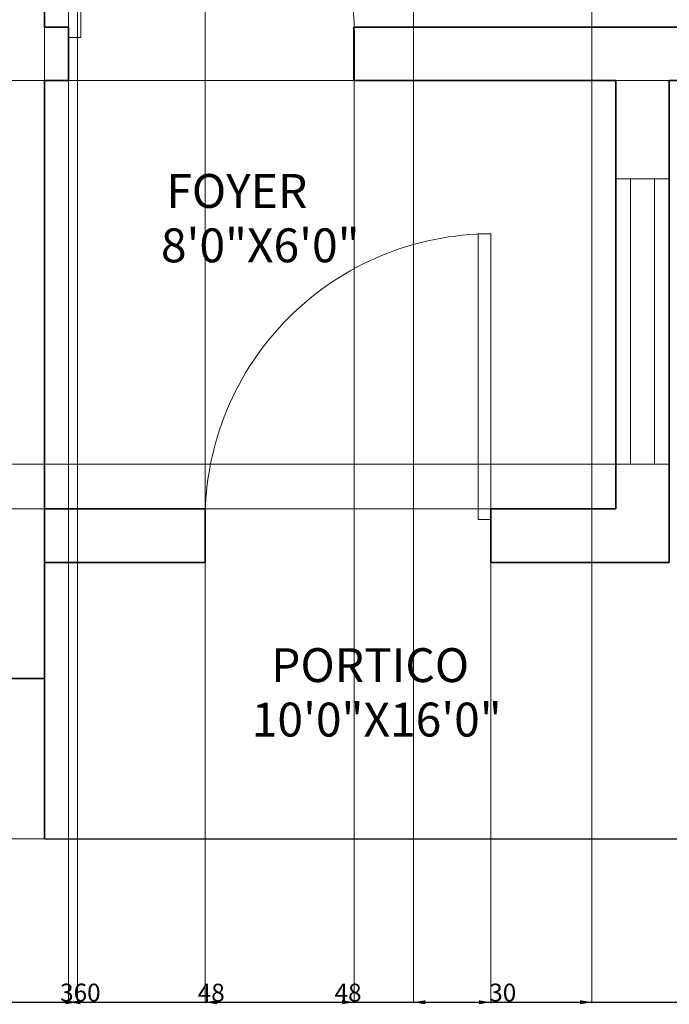
# Model space of a CAD drawing. Units: feet. Extents: x -297 to 770, y -228 to 625.
# Tile 3 of 14: x 552 to 661, y -228 to -62. Entities that reach past the tile are written whole.
import ezdxf

# ---------------------------------------------------------------- set-up
doc = ezdxf.new("R2010")
doc.units = ezdxf.units.FT
doc.header["$MEASUREMENT"] = 0
for name, color, linetype, lineweight in [('A-ANNO-DIMS', 2, 'Continuous', 18), ('A-AREA-IDEN', 7, 'Continuous', 25), ('A-FLOR-EDGE', 7, 'Continuous', 25), ('A-WALL', 7, 'Continuous', 35), ('doors', 30, 'Continuous', 18), ('windows', 30, 'Continuous', 18)]:
    doc.layers.add(name, color=color, linetype=linetype, lineweight=lineweight)
doc.styles.add('Annotative', font='arial.ttf')
doc.styles.get("Standard").update_dxf_attribs({"font": 'arial.ttf'})
doc.dimstyles.get("Standard").update_dxf_attribs({"dimtxt": 3, "dimasz": 2, "dimexe": 0.18, "dimexo": 0.0625, "dimgap": 0.09, "dimtad": 1, "dimtoh": 1, "dimdec": 1, "dimzin": 0, "dimdsep": 46, "dimlunit": 3, "dimtxsty": 'Standard', "dimcen": 0, "dimclre": 256, "dimadec": 0, "dimazin": 0, "dimtfac": 1, "dimtdec": 1, "dimtofl": 0, "dimtmove": 0, "dimatfit": 3, "dimfxl": 1, "dimtolj": 1, "dimtzin": 0, "dimlwe": -1, "dimarcsym": 0})

# ---------------------------------------------------------------- blocks, each defined once
blk = doc.blocks.new('*U5')
for p, q in [((-40, 0), (-40, 6)), ((0, 0), (0, 6))]:
    blk.add_line(p, q)
blk.add_lwpolyline([(0, 0), (0, -40), (-1.75, -40), (-1.75, 0)], close=True)
blk.add_arc((0, 0), 40, 180, 270)
blk = doc.blocks.new('*U4')
for p, q in [((0, 0), (0, 6)), ((40, 0), (40, 6))]:
    blk.add_line(p, q)
blk.add_lwpolyline([(0, 0), (0, -40), (1.75, -40), (1.75, 0)], close=True)
blk.add_arc((0, 0), 40, 270, 0)
blk = doc.blocks.new('WIN-4FT')
for p, q in [((48, 9), (0, 9)), ((0, 9), (0, 0)), ((48, 0), (48, 9)), ((0, 6.5), (48, 6.5)), ((0, 2.5), (48, 2.5)), ((0, 0), (48, 0))]:
    blk.add_line(p, q)
blk = doc.blocks.new('*D43')
at = {"layer": 'A-ANNO-DIMS', "transparency": 16777216}
for p, q in [((382.16, -173.1), (382.16, -227.67)), ((742.16, -200.1), (742.16, -227.67))]:
    blk.add_line(p, q, dxfattribs=at)
at = {"layer": 'A-ANNO-DIMS', "color": 0, "lineweight": -2, "transparency": 16777216}
blk.add_line((384.16, -227.49), (740.16, -227.49), dxfattribs=at)
at = {"layer": 'A-ANNO-DIMS', "color": 0, "transparency": 16777216}
for points in [[(384.16, -227.15), (384.16, -227.82), (382.16, -227.49)], [(740.16, -227.15), (740.16, -227.82), (742.16, -227.49)]]:
    blk.add_solid(points, dxfattribs=at)
at = {"layer": 'Defpoints', "color": 0, "transparency": 16777216}
for p in [(382.16, -173.04), (742.16, -200.04), (742.16, -227.49)]:
    blk.add_point(p, dxfattribs=at)
at = {"layer": 'A-ANNO-DIMS', "color": 0, "transparency": 16777216, "insert": (562.16, -225.86), "char_height": 3, "attachment_point": 5}
blk.add_mtext('\\A1;360', dxfattribs=at)
blk = doc.blocks.new('*D45')
at = {"layer": 'A-ANNO-DIMS', "transparency": 16777216}
for p, q in [((382.09, -173.04), (354.53, -173.04)), ((556.09, -200.04), (354.53, -200.04))]:
    blk.add_line(p, q, dxfattribs=at)
at = {"layer": 'A-ANNO-DIMS', "color": 0, "lineweight": -2, "transparency": 16777216}
blk.add_line((354.71, -175.04), (354.71, -198.04), dxfattribs=at)
at = {"layer": 'A-ANNO-DIMS', "color": 0, "transparency": 16777216}
for points in [[(354.37, -175.04), (355.04, -175.04), (354.71, -173.04)], [(354.37, -198.04), (355.04, -198.04), (354.71, -200.04)]]:
    blk.add_solid(points, dxfattribs=at)
at = {"layer": 'Defpoints', "color": 0, "transparency": 16777216}
for p in [(382.16, -173.04), (354.71, -200.04), (556.16, -200.04)]:
    blk.add_point(p, dxfattribs=at)
at = {"layer": 'A-ANNO-DIMS', "color": 0, "transparency": 16777216, "insert": (353.11, -186.54), "char_height": 3, "attachment_point": 5, "rotation": 90}
blk.add_mtext('\\A1;27', dxfattribs=at)
blk = doc.blocks.new('*D56')
at = {"layer": 'A-ANNO-DIMS', "transparency": 16777216}
for p, q in [((742.09, -72.54), (354.53, -72.54)), ((742.09, -200.04), (354.53, -200.04))]:
    blk.add_line(p, q, dxfattribs=at)
at = {"layer": 'A-ANNO-DIMS', "color": 0, "lineweight": -2, "transparency": 16777216}
blk.add_line((354.71, -74.54), (354.71, -198.04), dxfattribs=at)
at = {"layer": 'A-ANNO-DIMS', "color": 0, "transparency": 16777216}
for points in [[(354.37, -74.54), (355.04, -74.54), (354.71, -72.54)], [(354.37, -198.04), (355.04, -198.04), (354.71, -200.04)]]:
    blk.add_solid(points, dxfattribs=at)
at = {"layer": 'Defpoints', "color": 0, "transparency": 16777216}
for p in [(742.16, -72.54), (354.71, -200.04), (742.16, -200.04)]:
    blk.add_point(p, dxfattribs=at)
at = {"layer": 'A-ANNO-DIMS', "color": 0, "transparency": 16777216, "insert": (353.08, -136.29), "char_height": 3, "attachment_point": 5, "rotation": 90}
blk.add_mtext('\\A1;127.5', dxfattribs=at)
blk = doc.blocks.new('*D59')
at = {"layer": 'A-ANNO-DIMS', "transparency": 16777216}
for p, q in [((652.09, -137.04), (354.53, -137.04)), ((652.09, -144.54), (354.53, -144.54))]:
    blk.add_line(p, q, dxfattribs=at)
at = {"layer": 'A-ANNO-DIMS', "color": 0, "lineweight": -2, "transparency": 16777216}
blk.add_line((354.71, -142.54), (354.71, -139.04), dxfattribs=at)
at = {"layer": 'A-ANNO-DIMS', "color": 0, "transparency": 16777216}
for points in [[(354.37, -139.04), (355.04, -139.04), (354.71, -137.04)], [(354.37, -142.54), (355.04, -142.54), (354.71, -144.54)]]:
    blk.add_solid(points, dxfattribs=at)
at = {"layer": 'Defpoints', "color": 0, "transparency": 16777216}
for p in [(354.71, -137.04), (652.16, -137.04), (652.16, -144.54)]:
    blk.add_point(p, dxfattribs=at)
at = {"layer": 'A-ANNO-DIMS', "color": 0, "transparency": 16777216, "insert": (353.09, -140.79), "char_height": 3, "attachment_point": 5, "rotation": 90}
blk.add_mtext('\\A1;7.5', dxfattribs=at)
blk = doc.blocks.new('*D60')
at = {"layer": 'A-ANNO-DIMS', "transparency": 16777216}
for p, q in [((556.16, -144.47), (556.16, 367.22)), ((583.16, -144.47), (583.16, 367.22))]:
    blk.add_line(p, q, dxfattribs=at)
at = {"layer": 'A-ANNO-DIMS', "color": 0, "lineweight": -2, "transparency": 16777216}
blk.add_line((558.16, 367.04), (581.16, 367.04), dxfattribs=at)
at = {"layer": 'A-ANNO-DIMS', "color": 0, "transparency": 16777216}
for points in [[(558.16, 367.38), (558.16, 366.71), (556.16, 367.04)], [(581.16, 367.38), (581.16, 366.71), (583.16, 367.04)]]:
    blk.add_solid(points, dxfattribs=at)
at = {"layer": 'Defpoints', "color": 0, "transparency": 16777216}
for p in [(583.16, 367.04), (556.16, -144.54), (583.16, -144.54)]:
    blk.add_point(p, dxfattribs=at)
at = {"layer": 'A-ANNO-DIMS', "color": 0, "transparency": 16777216, "insert": (569.66, 368.64), "char_height": 3, "attachment_point": 5}
blk.add_mtext('\\A1;27', dxfattribs=at)
blk = doc.blocks.new('*D61')
at = {"layer": 'A-ANNO-DIMS', "transparency": 16777216}
for p, q in [((583.16, -153.6), (583.16, -227.67)), ((631.16, -153.6), (631.16, -227.67))]:
    blk.add_line(p, q, dxfattribs=at)
at = {"layer": 'A-ANNO-DIMS', "color": 0, "lineweight": -2, "transparency": 16777216}
blk.add_line((585.16, -227.49), (629.16, -227.49), dxfattribs=at)
at = {"layer": 'A-ANNO-DIMS', "color": 0, "transparency": 16777216}
for points in [[(585.16, -227.15), (585.16, -227.82), (583.16, -227.49)], [(629.16, -227.15), (629.16, -227.82), (631.16, -227.49)]]:
    blk.add_solid(points, dxfattribs=at)
at = {"layer": 'Defpoints', "color": 0, "transparency": 16777216}
for p in [(583.16, -153.54), (631.16, -153.54), (631.16, -227.49)]:
    blk.add_point(p, dxfattribs=at)
at = {"layer": 'A-ANNO-DIMS', "color": 0, "transparency": 16777216, "insert": (607.16, -225.87), "char_height": 3, "attachment_point": 5}
blk.add_mtext('\\A1;48', dxfattribs=at)
blk = doc.blocks.new('*D62')
at = {"layer": 'A-ANNO-DIMS', "transparency": 16777216}
for p, q in [((560.16, -72.6), (560.16, -227.67)), ((608.16, -72.6), (608.16, -227.67))]:
    blk.add_line(p, q, dxfattribs=at)
at = {"layer": 'A-ANNO-DIMS', "color": 0, "lineweight": -2, "transparency": 16777216}
blk.add_line((562.16, -227.49), (606.16, -227.49), dxfattribs=at)
at = {"layer": 'A-ANNO-DIMS', "color": 0, "transparency": 16777216}
for points in [[(562.16, -227.15), (562.16, -227.82), (560.16, -227.49)], [(606.16, -227.15), (606.16, -227.82), (608.16, -227.49)]]:
    blk.add_solid(points, dxfattribs=at)
at = {"layer": 'Defpoints', "color": 0, "transparency": 16777216}
for p in [(560.16, -72.54), (608.16, -72.54), (608.16, -227.49)]:
    blk.add_point(p, dxfattribs=at)
at = {"layer": 'A-ANNO-DIMS', "color": 0, "transparency": 16777216, "insert": (584.16, -225.87), "char_height": 3, "attachment_point": 5}
blk.add_mtext('\\A1;48', dxfattribs=at)
blk = doc.blocks.new('*D64')
at = {"layer": 'A-ANNO-DIMS', "transparency": 16777216}
for p, q in [((618.16, 233.4), (618.16, -227.67)), ((648.16, 233.4), (648.16, -227.67))]:
    blk.add_line(p, q, dxfattribs=at)
at = {"layer": 'A-ANNO-DIMS', "color": 0, "lineweight": -2, "transparency": 16777216}
blk.add_line((620.16, -227.49), (646.16, -227.49), dxfattribs=at)
at = {"layer": 'A-ANNO-DIMS', "color": 0, "transparency": 16777216}
for points in [[(620.16, -227.15), (620.16, -227.82), (618.16, -227.49)], [(646.16, -227.15), (646.16, -227.82), (648.16, -227.49)]]:
    blk.add_solid(points, dxfattribs=at)
at = {"layer": 'Defpoints', "color": 0, "transparency": 16777216}
for p in [(618.16, 233.46), (648.16, 233.46), (648.16, -227.49)]:
    blk.add_point(p, dxfattribs=at)
at = {"layer": 'A-ANNO-DIMS', "color": 0, "transparency": 16777216, "insert": (633.16, -225.86), "char_height": 3, "attachment_point": 5}
blk.add_mtext('\\A1;30', dxfattribs=at)
blk = doc.blocks.new('*D67')
at = {"layer": 'A-ANNO-DIMS', "transparency": 16777216}
for p, q in [((532.66, 197.4), (532.66, -227.67)), ((561.66, 197.4), (561.66, -227.67))]:
    blk.add_line(p, q, dxfattribs=at)
at = {"layer": 'A-ANNO-DIMS', "color": 0, "lineweight": -2, "transparency": 16777216}
blk.add_line((534.66, -227.49), (559.66, -227.49), dxfattribs=at)
at = {"layer": 'A-ANNO-DIMS', "color": 0, "transparency": 16777216}
for points in [[(534.66, -227.15), (534.66, -227.82), (532.66, -227.49)], [(559.66, -227.15), (559.66, -227.82), (561.66, -227.49)]]:
    blk.add_solid(points, dxfattribs=at)
at = {"layer": 'Defpoints', "color": 0, "transparency": 16777216}
for p in [(532.66, 197.46), (561.66, 197.46), (561.66, -227.49)]:
    blk.add_point(p, dxfattribs=at)
at = {"layer": 'A-ANNO-DIMS', "color": 0, "transparency": 16777216, "insert": (547.16, -225.87), "char_height": 3, "attachment_point": 5}
blk.add_mtext('\\A1;29', dxfattribs=at)

msp = doc.modelspace()

# ---------------------------------------------------------------- linework, layer by layer
at = {"layer": 'A-FLOR-EDGE'}
msp.add_line((556.155, -200.037), (742.155, -200.037), dxfattribs=at)
at = {"layer": 'A-WALL'}
for p, q in [((556.155, -63.537), (556.155, -45.037)), ((560.155, -63.537), (556.155, -63.537)), ((560.155, -63.537), (560.155, -72.537)), ((733.155, -63.537), (608.155, -63.537)), ((608.155, -63.537), (608.155, -72.537)), ((556.155, -72.537), (556.155, -200.037)), ((560.155, -72.537), (556.155, -72.537)), ((652.155, -72.537), (608.155, -72.537)), ((652.155, -72.537), (652.155, -144.537)), ((742.155, -72.537), (661.155, -72.537)), ((661.155, -72.537), (661.155, -153.537)), ((583.155, -144.537), (556.155, -144.537)), ((583.155, -144.537), (583.155, -153.537)), ((652.155, -144.537), (631.155, -144.537)), ((631.155, -144.537), (631.155, -153.537)), ((583.155, -153.537), (556.155, -153.537)), ((661.155, -153.537), (631.155, -153.537))]:
    msp.add_line(p, q, dxfattribs=at)
msp.add_lwpolyline([(685.155, 306.963), (382.155, 306.963), (382.155, -173.037), (556.155, -173.037)], dxfattribs=at)

# ---------------------------------------------------------------- block references
at = {"layer": 'doors', "rotation": 180}
for name, p, xscale, yscale, zscale in [('*U5', (560.155, -65.322), 1.202549277038201, 1.202549277038201, 1.202549277038201), ('*U4', (631.155, -146.334), 1.200582719259484, 1.200582719259484, 1.200582719259484)]:
    msp.add_blockref(name, p, dxfattribs=dict(at, xscale=xscale, yscale=yscale, zscale=zscale))
at = {"layer": 'windows', "rotation": 89.99999999999987}
msp.add_blockref('WIN-4FT', (661.155, -137.037), dxfattribs=at)

# ---------------------------------------------------------------- texts
at = {"layer": 'A-AREA-IDEN', "style": 'Annotative'}
for s, height, p in [('FOYER', 5.696, (576.619, -93.94)), ('8\'0"X6\'0"', 5.696, (575.705, -103.091)), ('PORTICO', 5.696, (594.237, -173.665)), (' 10\'0"X16\'0"', 5.69601, (589.23, -182.815))]:
    msp.add_text(s, height=height, dxfattribs=at).set_placement(p)

# ---------------------------------------------------------------- dimensions: what is measured, and where the dimension line sits
at = {"layer": 'A-ANNO-DIMS'}
for base, p1, p2, picture, middle in [((583.155, 367.042), (556.155, -144.537), (583.155, -144.537), '*D60', (569.655, 368.638)), ((648.155, -227.487), (618.155, 233.463), (648.155, 233.463), '*D64', (633.155, -225.865)), ((561.655, -227.487), (532.655, 197.463), (561.655, 197.463), '*D67', (547.155, -225.866)), ((608.155, -227.487), (560.155, -72.537), (608.155, -72.537), '*D62', (584.155, -225.866)), ((631.155, -227.487), (583.155, -153.537), (631.155, -153.537), '*D61', (607.155, -225.866)), ((742.155, -227.487), (382.155, -173.037), (742.155, -200.037), '*D43', (562.155, -225.865))]:
    dim = msp.add_linear_dim(base=base, p1=p1, p2=p2, dimstyle='Standard', override={"dimdec": 0, "dimlfac": 1, "dimrnd": 0, "dimzin": 0, "dimdsep": 46, "dimlunit": 2}, dxfattribs=at)
    dim.commit()
    dim.dimension.update_dxf_attribs({"geometry": picture, "text_midpoint": middle})
for base, p1, p2, override, picture, middle in [((354.705, -200.037), (742.155, -72.537), (742.155, -200.037), {"dimdec": 1, "dimlfac": 1, "dimrnd": 0, "dimzin": 0, "dimdsep": 46, "dimlunit": 2}, '*D56', (353.084, -136.287)), ((354.705, -137.037), (652.155, -144.537), (652.155, -137.037), {"dimdec": 1, "dimlfac": 1, "dimrnd": 0, "dimzin": 0, "dimdsep": 46, "dimlunit": 2}, '*D59', (353.09, -140.787)), ((354.705, -200.037), (382.155, -173.037), (556.155, -200.037), {"dimdec": 0, "dimlfac": 1, "dimrnd": 0, "dimzin": 0, "dimdsep": 46, "dimlunit": 2}, '*D45', (353.109, -186.537))]:
    dim = msp.add_linear_dim(base=base, p1=p1, p2=p2, angle=90, dimstyle='Standard', override=override, dxfattribs=at)
    dim.commit()
    dim.dimension.update_dxf_attribs({"geometry": picture, "text_midpoint": middle})

doc.saveas('drawing.dxf')
